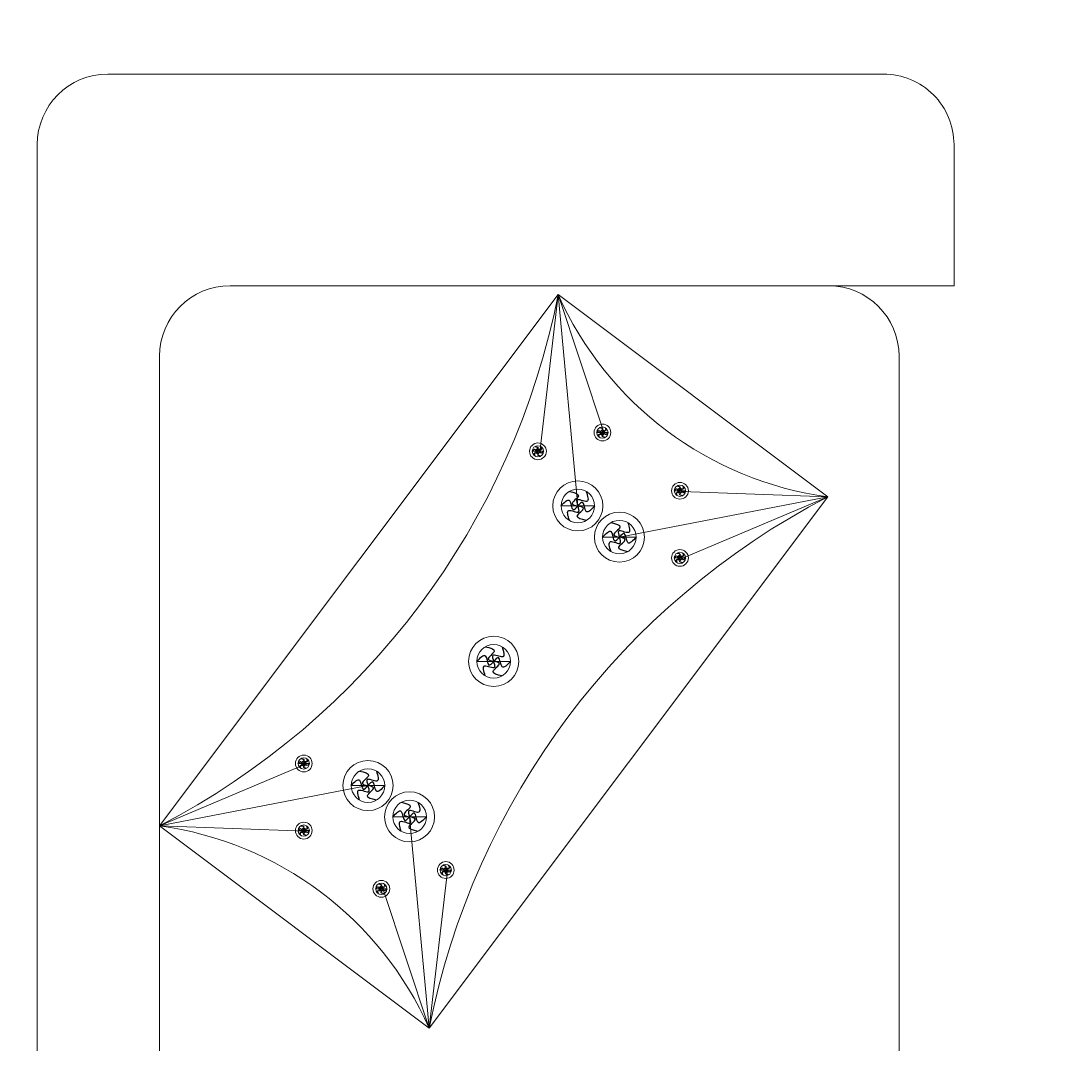
# Model space of a CAD drawing. Units: inches. Extents: x -61 to 1599, y -1316 to 257.
# Tile 131 of 204: x 388 to 418, y -106 to -77. Entities that reach past the tile are written whole.
import ezdxf

# ---------------------------------------------------------------- set-up
doc = ezdxf.new("R2010")
doc.units = ezdxf.units.IN
doc.header["$MEASUREMENT"] = 0
doc.layers.add('A-ANNO-DIMS', color=2, linetype='Continuous', lineweight=18)
doc.layers.add('FURNITURE', color=83, linetype='Continuous', lineweight=18)
doc.layers.add('FUR', color=83, linetype='Continuous')
doc.styles.get("Standard").update_dxf_attribs({"font": 'arial.ttf'})
doc.dimstyles.get("Standard").update_dxf_attribs({"dimtxt": 0.18, "dimasz": 0.18, "dimexe": 0.18, "dimexo": 0.0625, "dimgap": 0.09, "dimtad": 0, "dimtih": 1, "dimtoh": 1, "dimdec": 0, "dimzin": 0, "dimdsep": 46, "dimlunit": 3, "dimtxsty": 'Standard', "dimcen": 0.09, "dimadec": 0, "dimazin": 0, "dimtfac": 1, "dimtdec": 0, "dimtofl": 0, "dimtmove": 0, "dimatfit": 3, "dimfxl": 1, "dimtolj": 1, "dimtzin": 0, "dimarcsym": 0})

# ---------------------------------------------------------------- blocks, each defined once
blk = doc.blocks.new('*U186')
at = {"layer": 'FUR'}
blk.add_open_spline([(0.005, 0.08), (-0.03, 0.048), (-0.098, -0.015), (0.075, -0.018), (0.024, -0.063), (0.005, -0.08)], degree=3, knots=[0, 0, 0, 0, 0.0954578, 0.1898773, 0.2470677, 0.2470677, 0.2470677, 0.2470677], dxfattribs=at)
blk = doc.blocks.new('*U187')
at = {"layer": 'FUR', "transparency": 16777216}
for p, rotation in [((222.173, -79.977), 60), ((222.178, -80.056), 120), ((222.25, -80.092), 180), ((222.312, -79.968), 300), ((222.317, -80.048), 240)]:
    blk.add_blockref('*U186', p, dxfattribs=dict(at, rotation=rotation))
blk.add_blockref('*U186', (222.24, -79.932), dxfattribs=at)
blk = doc.blocks.new('*U198')
at = {"layer": 'FUR'}
blk.add_open_spline([(0.005, 0.08), (-0.03, 0.048), (-0.098, -0.015), (0.075, -0.018), (0.024, -0.063), (0.005, -0.08)], degree=3, knots=[0, 0, 0, 0, 0.0954578, 0.1898773, 0.2470677, 0.2470677, 0.2470677, 0.2470677], dxfattribs=at)
blk = doc.blocks.new('*U199')
at = {"layer": 'FUR', "transparency": 16777216}
for p, rotation in [((222.173, -79.977), 60), ((222.178, -80.056), 120), ((222.25, -80.092), 180), ((222.312, -79.968), 300), ((222.317, -80.048), 240)]:
    blk.add_blockref('*U198', p, dxfattribs=dict(at, rotation=rotation))
blk.add_blockref('*U198', (222.24, -79.932), dxfattribs=at)
blk = doc.blocks.new('*U210')
at = {"layer": 'FUR'}
blk.add_open_spline([(0.015, 0.238), (-0.088, 0.143), (-0.292, -0.045), (0.224, -0.053), (0.072, -0.187), (0.015, -0.238)], degree=3, knots=[0, 0, 0, 0, 0.2846533, 0.5662105, 0.736751, 0.736751, 0.736751, 0.736751], dxfattribs=at)
blk = doc.blocks.new('*U185')
at = {"layer": 'FUR', "transparency": 16777216}
blk.add_blockref('*U210', (662.716, -238.357), dxfattribs=at)
for p, rotation in [((662.929, -238.463), 300), ((662.517, -238.489), 60), ((662.531, -238.727), 120), ((662.944, -238.702), 240), ((662.745, -238.833), 180)]:
    blk.add_blockref('*U210', p, dxfattribs=dict(at, rotation=rotation))
blk = doc.blocks.new('*U200')
at = {"layer": 'FUR'}
blk.add_open_spline([(0.005, 0.08), (-0.03, 0.048), (-0.098, -0.015), (0.075, -0.018), (0.024, -0.063), (0.005, -0.08)], degree=3, knots=[0, 0, 0, 0, 0.0954578, 0.1898773, 0.2470677, 0.2470677, 0.2470677, 0.2470677], dxfattribs=at)
blk = doc.blocks.new('*U201')
at = {"layer": 'FUR', "transparency": 16777216}
for p, rotation in [((222.173, -79.977), 60), ((222.178, -80.056), 120), ((222.25, -80.092), 180), ((222.312, -79.968), 300), ((222.317, -80.048), 240)]:
    blk.add_blockref('*U200', p, dxfattribs=dict(at, rotation=rotation))
blk.add_blockref('*U200', (222.24, -79.932), dxfattribs=at)
blk = doc.blocks.new('*U194')
at = {"layer": 'FUR'}
blk.add_open_spline([(0.015, 0.238), (-0.088, 0.143), (-0.292, -0.045), (0.224, -0.053), (0.072, -0.187), (0.015, -0.238)], degree=3, knots=[0, 0, 0, 0, 0.2846533, 0.5662105, 0.736751, 0.736751, 0.736751, 0.736751], dxfattribs=at)
blk = doc.blocks.new('*U195')
at = {"layer": 'FUR', "transparency": 16777216}
blk.add_blockref('*U194', (662.716, -238.357), dxfattribs=at)
for p, rotation in [((662.929, -238.463), 300), ((662.517, -238.489), 60), ((662.531, -238.727), 120), ((662.944, -238.702), 240), ((662.745, -238.833), 180)]:
    blk.add_blockref('*U194', p, dxfattribs=dict(at, rotation=rotation))
blk = doc.blocks.new('*U202')
at = {"layer": 'FUR'}
blk.add_open_spline([(0.005, 0.08), (-0.03, 0.048), (-0.098, -0.015), (0.075, -0.018), (0.024, -0.063), (0.005, -0.08)], degree=3, knots=[0, 0, 0, 0, 0.0954578, 0.1898773, 0.2470677, 0.2470677, 0.2470677, 0.2470677], dxfattribs=at)
blk = doc.blocks.new('*U203')
at = {"layer": 'FUR', "transparency": 16777216}
for p, rotation in [((222.173, -79.977), 60), ((222.178, -80.056), 120), ((222.25, -80.092), 180), ((222.312, -79.968), 300), ((222.317, -80.048), 240)]:
    blk.add_blockref('*U202', p, dxfattribs=dict(at, rotation=rotation))
blk.add_blockref('*U202', (222.24, -79.932), dxfattribs=at)
blk = doc.blocks.new('*U196')
at = {"layer": 'FUR'}
blk.add_open_spline([(0.015, 0.238), (-0.088, 0.143), (-0.292, -0.045), (0.224, -0.053), (0.072, -0.187), (0.015, -0.238)], degree=3, knots=[0, 0, 0, 0, 0.2846533, 0.5662105, 0.736751, 0.736751, 0.736751, 0.736751], dxfattribs=at)
blk = doc.blocks.new('*U197')
at = {"layer": 'FUR', "transparency": 16777216}
blk.add_blockref('*U196', (662.716, -238.357), dxfattribs=at)
for p, rotation in [((662.929, -238.463), 300), ((662.517, -238.489), 60), ((662.531, -238.727), 120), ((662.944, -238.702), 240), ((662.745, -238.833), 180)]:
    blk.add_blockref('*U196', p, dxfattribs=dict(at, rotation=rotation))
blk = doc.blocks.new('*U190')
at = {"layer": 'FUR'}
blk.add_open_spline([(0.005, 0.08), (-0.03, 0.048), (-0.098, -0.015), (0.075, -0.018), (0.024, -0.063), (0.005, -0.08)], degree=3, knots=[0, 0, 0, 0, 0.0954578, 0.1898773, 0.2470677, 0.2470677, 0.2470677, 0.2470677], dxfattribs=at)
blk = doc.blocks.new('*U191')
at = {"layer": 'FUR', "transparency": 16777216}
for p, rotation in [((222.173, -79.977), 60), ((222.178, -80.056), 120), ((222.25, -80.092), 180), ((222.312, -79.968), 300), ((222.317, -80.048), 240)]:
    blk.add_blockref('*U190', p, dxfattribs=dict(at, rotation=rotation))
blk.add_blockref('*U190', (222.24, -79.932), dxfattribs=at)
blk = doc.blocks.new('*U209')
at = {"layer": 'FUR'}
blk.add_open_spline([(0.015, 0.238), (-0.088, 0.143), (-0.292, -0.045), (0.224, -0.053), (0.072, -0.187), (0.015, -0.238)], degree=3, knots=[0, 0, 0, 0, 0.2846533, 0.5662105, 0.736751, 0.736751, 0.736751, 0.736751], dxfattribs=at)
blk = doc.blocks.new('*U188')
at = {"layer": 'FUR', "transparency": 16777216}
blk.add_blockref('*U209', (662.716, -238.357), dxfattribs=at)
for p, rotation in [((662.929, -238.463), 300), ((662.517, -238.489), 60), ((662.531, -238.727), 120), ((662.944, -238.702), 240), ((662.745, -238.833), 180)]:
    blk.add_blockref('*U209', p, dxfattribs=dict(at, rotation=rotation))
blk = doc.blocks.new('*U208')
at = {"layer": 'FUR'}
blk.add_open_spline([(0.005, 0.08), (-0.03, 0.048), (-0.098, -0.015), (0.075, -0.018), (0.024, -0.063), (0.005, -0.08)], degree=3, knots=[0, 0, 0, 0, 0.0954578, 0.1898773, 0.2470677, 0.2470677, 0.2470677, 0.2470677], dxfattribs=at)
blk = doc.blocks.new('*U189')
at = {"layer": 'FUR', "transparency": 16777216}
for p, rotation in [((222.173, -79.977), 60), ((222.178, -80.056), 120), ((222.25, -80.092), 180), ((222.312, -79.968), 300), ((222.317, -80.048), 240)]:
    blk.add_blockref('*U208', p, dxfattribs=dict(at, rotation=rotation))
blk.add_blockref('*U208', (222.24, -79.932), dxfattribs=at)
blk = doc.blocks.new('*U192')
at = {"layer": 'FUR'}
blk.add_open_spline([(0.015, 0.238), (-0.088, 0.143), (-0.292, -0.045), (0.224, -0.053), (0.072, -0.187), (0.015, -0.238)], degree=3, knots=[0, 0, 0, 0, 0.2846533, 0.5662105, 0.736751, 0.736751, 0.736751, 0.736751], dxfattribs=at)
blk = doc.blocks.new('*U193')
at = {"layer": 'FUR', "transparency": 16777216}
blk.add_blockref('*U192', (662.716, -238.357), dxfattribs=at)
for p, rotation in [((662.929, -238.463), 300), ((662.517, -238.489), 60), ((662.531, -238.727), 120), ((662.944, -238.702), 240), ((662.745, -238.833), 180)]:
    blk.add_blockref('*U192', p, dxfattribs=dict(at, rotation=rotation))
blk = doc.blocks.new('*U204')
at = {"layer": 'FUR'}
blk.add_open_spline([(0.005, 0.08), (-0.03, 0.048), (-0.098, -0.015), (0.075, -0.018), (0.024, -0.063), (0.005, -0.08)], degree=3, knots=[0, 0, 0, 0, 0.0954578, 0.1898773, 0.2470677, 0.2470677, 0.2470677, 0.2470677], dxfattribs=at)
blk = doc.blocks.new('*U205')
at = {"layer": 'FUR', "transparency": 16777216}
for p, rotation in [((222.173, -79.977), 60), ((222.178, -80.056), 120), ((222.25, -80.092), 180), ((222.312, -79.968), 300), ((222.317, -80.048), 240)]:
    blk.add_blockref('*U204', p, dxfattribs=dict(at, rotation=rotation))
blk.add_blockref('*U204', (222.24, -79.932), dxfattribs=at)
blk = doc.blocks.new('*U206')
at = {"layer": 'FUR'}
blk.add_open_spline([(0.005, 0.08), (-0.03, 0.048), (-0.098, -0.015), (0.075, -0.018), (0.024, -0.063), (0.005, -0.08)], degree=3, knots=[0, 0, 0, 0, 0.0954578, 0.1898773, 0.2470677, 0.2470677, 0.2470677, 0.2470677], dxfattribs=at)
blk = doc.blocks.new('*U207')
at = {"layer": 'FUR', "transparency": 16777216}
for p, rotation in [((222.173, -79.977), 60), ((222.178, -80.056), 120), ((222.25, -80.092), 180), ((222.312, -79.968), 300), ((222.317, -80.048), 240)]:
    blk.add_blockref('*U206', p, dxfattribs=dict(at, rotation=rotation))
blk.add_blockref('*U206', (222.24, -79.932), dxfattribs=at)
blk = doc.blocks.new('SOFA-LOVESEAT')
for p, q in [((22.442, 54), (5.47, 54)), ((22.442, 54), (26, 54)), ((14.776, 53.751), (14.253, 49.285)), ((14.776, 53.751), (15.332, 47.757)), ((14.776, 53.751), (16.081, 49.817)), ((3.47, 8), (3.47, 52)), ((24.442, 52), (24.442, 32)), ((16.029, 49.837), (15.869, 49.837)), ((16.029, 49.837), (16.189, 49.837)), ((14.201, 49.305), (14.041, 49.305)), ((14.201, 49.305), (14.36, 49.305)), ((22.422, 48.013), (16.511, 46.872)), ((18.228, 48.187), (18.068, 48.187)), ((18.228, 48.187), (18.388, 48.187)), ((22.422, 48.013), (18.28, 48.167)), ((22.422, 48.013), (18.28, 46.263)), ((15.332, 47.757), (14.855, 47.757)), ((15.332, 47.757), (15.808, 47.757)), ((16.511, 46.872), (16.035, 46.872)), ((16.511, 46.872), (16.988, 46.872)), ((18.228, 46.282), (18.068, 46.282)), ((18.228, 46.282), (18.388, 46.282)), ((12.946, 43.35), (12.47, 43.35)), ((12.946, 43.35), (13.423, 43.35)), ((3.47, 38.686), (7.612, 40.436)), ((7.56, 40.455), (7.4, 40.455)), ((7.56, 40.455), (7.719, 40.455)), ((3.47, 38.686), (9.381, 39.828)), ((9.381, 39.828), (8.904, 39.828)), ((9.381, 39.828), (9.857, 39.828)), ((10.561, 38.942), (10.084, 38.942)), ((11.116, 32.948), (10.561, 38.942)), ((10.561, 38.942), (11.037, 38.942)), ((3.47, 38.686), (7.612, 38.532)), ((7.56, 38.551), (7.4, 38.551)), ((7.56, 38.551), (7.719, 38.551)), ((11.116, 32.948), (11.639, 37.414)), ((11.587, 37.433), (11.427, 37.433)), ((11.587, 37.433), (11.747, 37.433)), ((9.759, 36.901), (9.599, 36.901)), ((9.759, 36.901), (9.918, 36.901)), ((11.116, 32.948), (9.811, 36.882))]:
    blk.add_line(p, q)
blk.add_lwpolyline([(26, 6), (26, 2, -0.414214), (24, 0), (2, 0, -0.414214), (0, 2), (0, 58, -0.414213), (2, 60), (24, 60, -0.414214), (26, 58), (26, 54)], format="xyb")
blk.add_lwpolyline([(11.116, 32.948), (22.422, 48.013), (14.776, 53.751), (3.47, 38.686)], close=True)
for centre, radius in [((16.029, 49.837), 0.238), ((16.029, 49.837), 0.16), ((14.201, 49.305), 0.238), ((14.201, 49.305), 0.16), ((15.332, 47.757), 0.71), ((18.228, 48.187), 0.238), ((18.228, 48.187), 0.16), ((15.332, 47.757), 0.476), ((16.511, 46.872), 0.71), ((16.511, 46.872), 0.476), ((18.228, 46.282), 0.238), ((18.228, 46.282), 0.16), ((12.946, 43.35), 0.71), ((12.946, 43.35), 0.476), ((7.56, 40.455), 0.238), ((7.56, 40.455), 0.16), ((9.381, 39.828), 0.71), ((9.381, 39.828), 0.476), ((10.561, 38.942), 0.71), ((10.561, 38.942), 0.476), ((7.56, 38.551), 0.238), ((7.56, 38.551), 0.16), ((11.587, 37.433), 0.238), ((11.587, 37.433), 0.16), ((9.759, 36.901), 0.238), ((9.759, 36.901), 0.16)]:
    blk.add_circle(centre, radius)
for centre, radius, start, end in [((5.47, 52), 2, 90, 180), ((22.442, 52), 2, 0, 90), ((-6.541, 57.974), 21.731, 297.4317, 348.7956), ((23.745, 57.74), 9.816, 203.9742, 262.253), ((32.433, 28.726), 21.731, 117.4317, 168.7956), ((2.147, 28.96), 9.816, 23.9742, 82.253)]:
    blk.add_arc(centre, radius, start, end)
at = {"xscale": -1, "rotation": 90.00003000000098}
for name, p in [('*U189', (-63.984, 272.082)), ('*U191', (-65.812, 271.55)), ('*U188', (-223.264, 710.487)), ('*U205', (-61.785, 270.431)), ('*U193', (-222.084, 709.602)), ('*U207', (-61.785, 268.527)), ('*U197', (-225.649, 706.08)), ('*U187', (-72.453, 262.7)), ('*U185', (-229.215, 702.558)), ('*U195', (-228.035, 701.672)), ('*U199', (-72.453, 260.796)), ('*U203', (-68.426, 259.678)), ('*U201', (-70.254, 259.146))]:
    blk.add_blockref(name, p, dxfattribs=at)
blk = doc.blocks.new('*D703')
at = {"layer": 'A-ANNO-DIMS', "color": 0, "lineweight": -2, "transparency": 16777216}
for p, q in [((372.32, -616.882), (372.32, 257.457)), ((372.5, 257.277), (413.7, 257.277)), ((455.653, 257.277), (414.453, 257.277)), ((455.833, -616.882), (455.833, 257.457))]:
    blk.add_line(p, q, dxfattribs=at)
at = {"layer": 'A-ANNO-DIMS', "color": 0, "transparency": 16777216}
for points in [[(372.5, 257.307), (372.5, 257.247), (372.32, 257.277)], [(455.653, 257.307), (455.653, 257.247), (455.833, 257.277)]]:
    blk.add_solid(points, dxfattribs=at)
at = {"layer": 'DEFPOINTS', "color": 0, "transparency": 16777216}
for p in [(455.833, 257.277), (372.32, -616.945), (455.833, -616.945)]:
    blk.add_point(p, dxfattribs=at)
at = {"layer": 'A-ANNO-DIMS', "color": 0, "transparency": 16777216, "insert": (414.076, 257.277), "char_height": 0.18, "attachment_point": 5}
blk.add_mtext('\\A1;83.51', dxfattribs=at)

msp = doc.modelspace()

# ---------------------------------------------------------------- block references
at = {"layer": 'FURNITURE'}
msp.add_blockref('SOFA-LOVESEAT', (388.9518, -138.383), dxfattribs=at)

# ---------------------------------------------------------------- dimensions: what is measured, and where the dimension line sits
at = {"layer": 'A-ANNO-DIMS'}
dim = msp.add_linear_dim(base=(455.8327, 257.2771), p1=(372.3201, -616.9446), p2=(455.8327, -616.9446), dimstyle='Standard', override={"dimdec": 2, "dimlfac": 1, "dimrnd": 0, "dimzin": 0, "dimdsep": 46, "dimlunit": 2}, dxfattribs=at)
dim.commit()
dim.dimension.update_dxf_attribs({"geometry": '*D703', "text_midpoint": (414.0764, 257.2771)})

doc.saveas('drawing.dxf')
